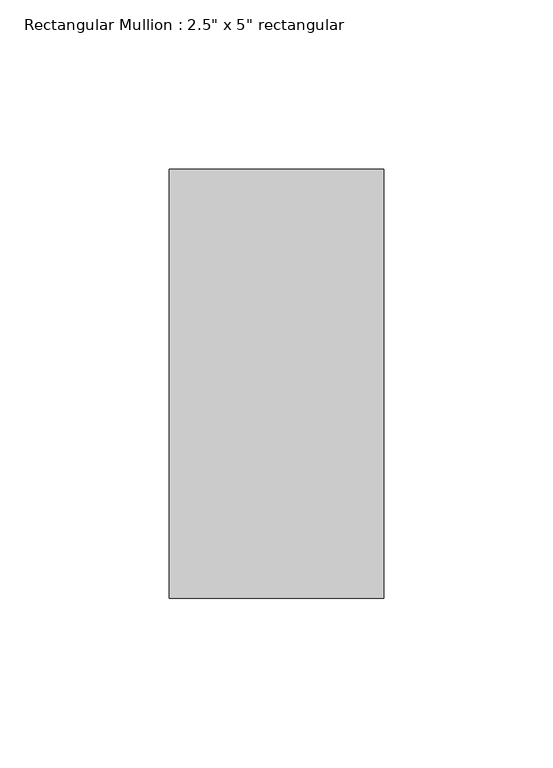
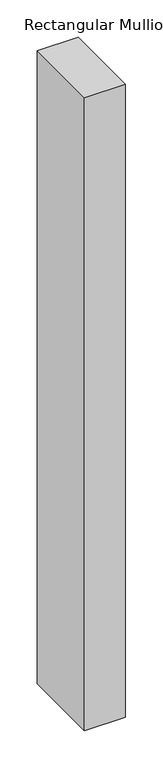
"""IFC4 building model written with IfcOpenShell, lengths in millimetres: member geometry."""

from ifc_helpers import new_model, si_unit, frame, origin, place, context, project, spatial, polyline, outline, extrude, source, transform, mapped, element, save


def member_3e299884(model_context):
    return source(origin(), model_context, "Body", "SweptSolid", [
        extrude(outline(polyline([(0.0, 63.5), (0.0, -63.5), (-63.5, -63.5), (-63.5, 63.5), (0.0, 63.5)])), frame((0.0, 0.0, -1038.9), z_axis=(0.0, 0.0, 1.0), x_axis=(1.0, 0.0, 0.0)), (0.0, 0.0, 1.0), 1038.9),
    ])


if __name__ == "__main__":
    model = new_model("IFC4")
    model_context = context("Model", 3, world=origin())
    ifc_project = project(units=[si_unit("LENGTHUNIT", "METRE", prefix="MILLI")], contexts=[model_context])
    site = spatial("IfcSite", under=ifc_project)
    building = spatial("IfcBuilding", under=site)
    placement = place(None, origin())
    member_shape = member_3e299884(model_context)
    element("IfcMember", 1, ObjectType="Rectangular Mullion : 2.5\" x 5\" rectangular", at=placement, inside=building, context=model_context, shape_type="MappedRepresentation", body=[
        mapped(member_shape, transform((0.0, 0.0, 0.0), x_axis=(1.0, 0.0, 0.0), y_axis=(0.0, 1.0, 0.0), z_axis=(0.0, 0.0, 1.0))),
    ])
    save(model, "model.ifc")

# Revit data of these elements
# Type "Rectangular Mullion : 2.5\" x 5\" rectangular"
#   built-in parameter 1007304 = 0.416667 (stored number, unit not read)
#   built-in parameter 1007301 = 0.104167 (stored number, unit not read)
#   built-in parameter 1007300 = 0.104167 (stored number, unit not read)
# Element 1 (IfcMember, "Rectangular Mullion : 2.5\" x 5\" rectangular")
#   Materials on its faces: "Damp-proofing"
# Materials
#   "Damp-proofing": class "Generic", colour RGB 127 127 127, transparency 0, Description = "Damp-proofing", Cost = 0
